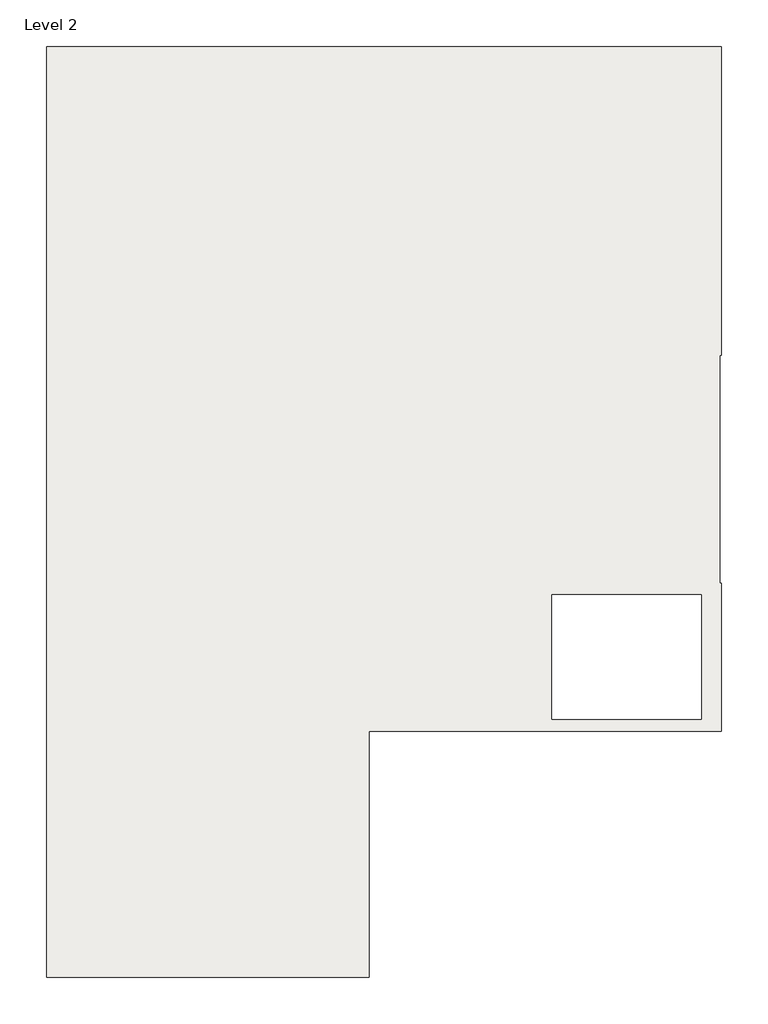
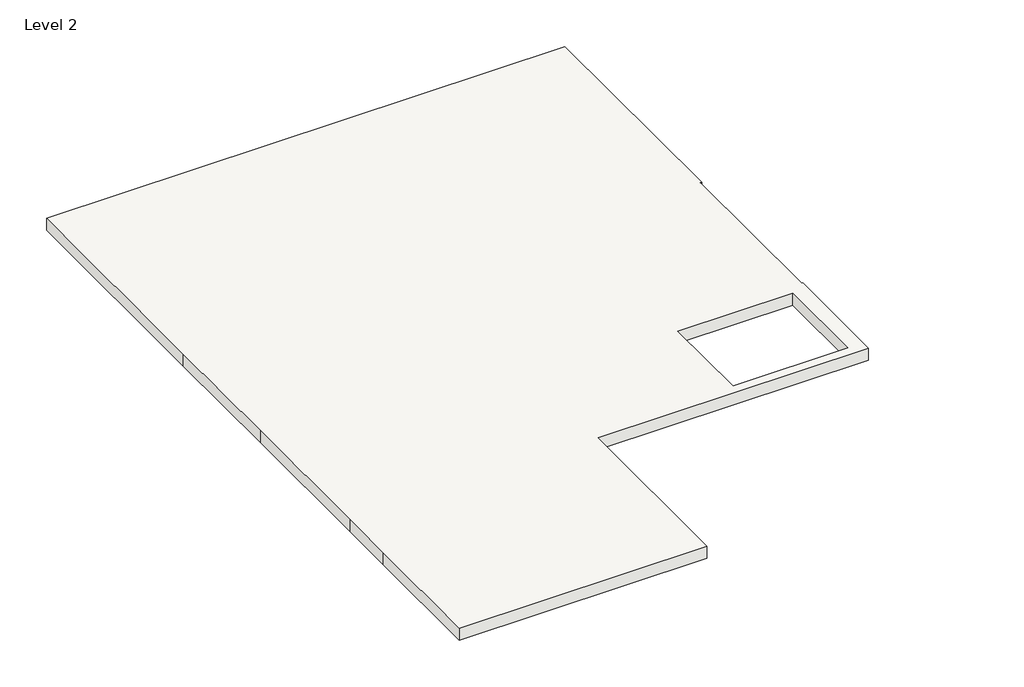
# One storey: 1 roof.
"""IFC4 building model written with IfcOpenShell, lengths in millimetres."""

from ifc_helpers import new_model, si_unit, frame, origin, place, context, project, spatial, polyline, outline, extrude, element, save

model = new_model("IFC4")

# Units and contexts
model_context = context("Model", 3, world=origin())
ifc_project = project(units=[si_unit("LENGTHUNIT", "METRE", prefix="MILLI")], contexts=[model_context])

# Site, building, storey
site = spatial("IfcSite", under=ifc_project)
building = spatial("IfcBuilding", under=site)
storey = spatial("IfcBuildingStorey", under=building, Name="Level 2", Elevation=3048.0)

# Roof
placement = place(None, origin())
element("IfcRoof", 1, ObjectType="Generic - 12\"", at=placement, inside=storey, context=model_context, shape_type="SweptSolid", body=[
    extrude(outline(polyline([(-14607.1841185, 13853.2271763), (-2211.9841185, 13853.2271763), (-2211.9841185, 8189.0271763), (-2237.3841185, 8189.0271763), (-2237.3841185, 3998.0271763), (-2211.9841185, 3998.0271763), (-2211.9841185, 1280.2271763), (-8682.6341185, 1280.2271763), (-8682.6341185, -3240.9728237), (-14607.1841185, -3240.9728237), (-14607.1841185, -91.3728237), (-14607.1841185, 1280.2271763), (-14607.1841185, 4988.6271763), (-14607.1841185, 8189.0271763), (-14607.1841185, 13853.2271763)]), holes=[polyline([(-2576.3100418, 1499.5155074), (-2576.3100418, 3785.5155074), (-5319.5100418, 3785.5155074), (-5319.5100418, 1499.5155074), (-2576.3100418, 1499.5155074)])]), frame((0.0, 0.0, 3048.0), z_axis=(0.0, 0.0, 1.0), x_axis=(1.0, 0.0, 0.0)), (0.0, 0.0, 1.0), 304.8),
])

save(model, "model.ifc")

# Revit data of these elements
# Type "Generic - 12\""
#   Assembly Code = "B1020"
#   Layers, outside or top first: 1' - 0" "Brick, Soldier Course" (function 1)
# Element 1 (IfcRoof, "Generic - 12\"")
#   built-in parameter 1001705 = 11 (stored number, unit not read)
#   built-in parameter 1001710 = 33615
#   Phase Created = New Construction
#   Materials on its faces: "Brick, Soldier Course"
# Materials
#   "Brick, Soldier Course": class "Masonry", colour RGB 170 98 104, transparency 0, Description = "Common brick soldier coursed", Cost = 0
